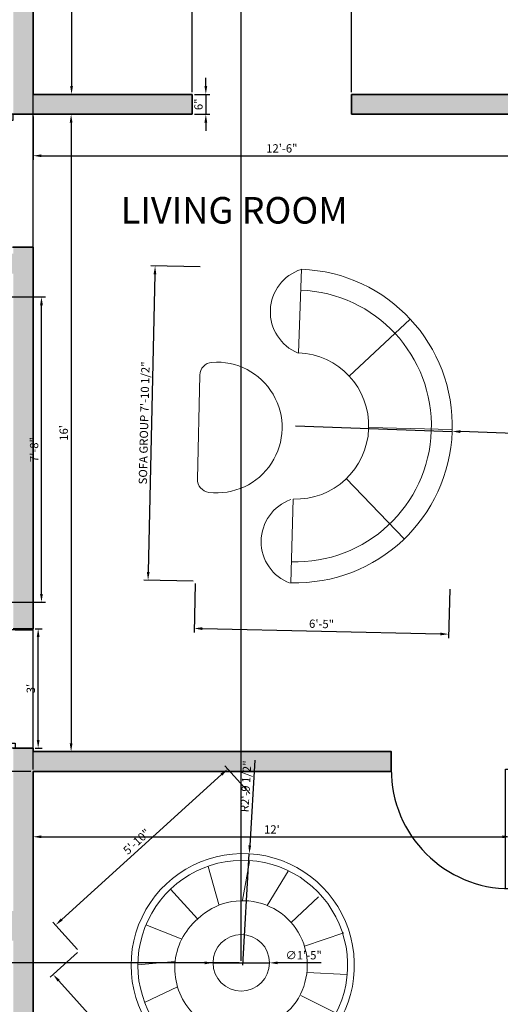
# Model space of a CAD drawing. Units: inches. Extents: x 2901 to 5923, y 918 to 2827.
# Tile 10 of 16: x 4585 to 4730, y 1227 to 1524. Entities that reach past the tile are written whole.
import ezdxf

# ---------------------------------------------------------------- set-up
doc = ezdxf.new("R2010")
doc.units = ezdxf.units.IN
for name, color, linetype, lineweight in [('A-ANNO-DIMS', 2, 'Continuous', 18), ('A-AREA-IDEN', 7, 'Continuous', 25), ('A-FLOR-PATT', 252, 'Continuous', 13), ('A-WALL-PATT', 7, 'Continuous', 13), ('doors', 240, 'Continuous', 25), ('furniture', 160, 'Continuous', 18), ('walls', 7, 'Continuous', 35)]:
    doc.layers.add(name, color=color, linetype=linetype, lineweight=lineweight)
doc.styles.get("Standard").update_dxf_attribs({"font": 'arial.ttf'})
doc.dimstyles.new('Copy of ISO-25', dxfattribs={"dimtxt": 2.5, "dimasz": 2.5, "dimexe": 1.25, "dimexo": 0.625, "dimtad": 1, "dimdec": 1, "dimlunit": 4, "dimtxsty": 'Standard', "dimcen": 2.5, "dimadec": 0, "dimazin": 0, "dimtfac": 1, "dimtdec": 1, "dimtmove": 0, "dimatfit": 3, "dimfxl": 1, "dimarcsym": 0})

# ---------------------------------------------------------------- blocks, each defined once
blk = doc.blocks.new('*U9')
for p, q in [((-40, 0), (-40, 6)), ((0, 0), (0, 6))]:
    blk.add_line(p, q)
blk.add_lwpolyline([(0, 0), (0, -40), (-1.75, -40), (-1.75, 0)], close=True)
blk.add_arc((0, 0), 40, 180, 270)
blk = doc.blocks.new('*U5')
for p, q in [((0, 0), (0, -6)), ((-40, 0), (-40, -6))]:
    blk.add_line(p, q)
blk.add_lwpolyline([(0, 0), (0, 40), (-1.75, 40), (-1.75, 0)], close=True)
blk.add_arc((0, 0), 40, 90, 180)
blk = doc.blocks.new('*U6')
for p, q in [((0, 0), (0, -6)), ((40, 0), (40, -6))]:
    blk.add_line(p, q)
blk.add_lwpolyline([(0, 0), (0, 40), (1.75, 40), (1.75, 0)], close=True)
blk.add_arc((0, 0), 40, 0, 90)
blk = doc.blocks.new('A$C22FC404C')
for p, q in [((1199.9, 1301.9), (1199.9, 1941.9)), ((809.2, 1143.1), (362.7, 1601.6)), ((1594.3, 1139.4), (2045.1, 1593.7)), ((0, 760.4), (639.9, 750.6)), ((2399.8, 731.4), (1759.8, 735.4)), ((827.3, 0), (1623.4, 0))]:
    blk.add_line(p, q)
for centre, radius, start, end in [((1199.9, 741.9), 1200, 359.49903, 179.11736), ((1199.9, 741.9), 1040, 359.40957, 179.11736), ((1199.9, 741.9), 560, 359.32862, 179.11736), ((323.1, 869.6), 340.6, 199.13086, 339.10386), ((2082.3, 838.8), 340.6, 200.89614, 340.86914), ((1225.3, 139.3), 500, 354.35827, 185.64173), ((827.3, 100), 100, 185.64173, 270), ((1623.4, 100), 100, 270, 354.35827)]:
    blk.add_arc(centre, radius, start, end)
blk = doc.blocks.new('A$C0ECE726C')
for p, q in [((1694, 2620), (1694, 3331)), ((1322, 2571), (1110, 3122)), ((1023, 2382), (606, 2799)), ((787, 2067), (221, 2311)), ((701, 1673), (142, 1666)), ((2687, 1673), (3320, 1664)), ((795, 1248), (221, 1075)), ((2593, 1248), (3113, 1091)), ((1016, 941), (551, 587)), ((2372, 941), (2811, 607)), ((1315, 753), (1055, 225)), ((2073, 753), (2322, 247)), ((1694, 100), (1694, 697))]:
    blk.add_line(p, q)
blk.add_circle((1652, 1618), 420)
for centre, radius, start, end in [((1660, 1660), 1660, 88.7606, 0.1441), ((1660, 1660), 1560, 88.7606, 0.2051), ((1392, 2970), 462, 310.7368, 49.2632), ((1660, 1660), 960, 87.986, 272.014), ((3002, 1543), 340, 20.831, 157.5545), ((1728, 1660), 960, 267.986, 0.781)]:
    blk.add_arc(centre, radius, start, end)
blk = doc.blocks.new('*D38')
at = {"layer": 'A-ANNO-DIMS', "color": 0, "lineweight": -2, "transparency": 16777216}
for p, q in [((4589.69, 1621.4), (4601.92, 1621.4)), ((4600.67, 1618.9), (4600.67, 1503.9)), ((4589.69, 1501.4), (4601.92, 1501.4))]:
    blk.add_line(p, q, dxfattribs=at)
at = {"layer": 'A-ANNO-DIMS', "color": 0, "transparency": 16777216}
for points in [[(4600.25, 1618.9), (4601.08, 1618.9), (4600.67, 1621.4)], [(4600.25, 1503.9), (4601.08, 1503.9), (4600.67, 1501.4)]]:
    blk.add_solid(points, dxfattribs=at)
at = {"layer": 'Defpoints', "color": 0, "transparency": 16777216}
for p in [(4589.07, 1621.4), (4589.07, 1501.4), (4600.67, 1501.4)]:
    blk.add_point(p, dxfattribs=at)
at = {"layer": 'A-ANNO-DIMS', "color": 0, "transparency": 16777216, "insert": (4598.76, 1561.4), "char_height": 2.5, "attachment_point": 5, "rotation": 90}
blk.add_mtext("10'", dxfattribs=at)
blk = doc.blocks.new('*D43')
at = {"layer": 'A-ANNO-DIMS', "color": 0, "lineweight": -2, "transparency": 16777216}
for p, q in [((4589.69, 1340.4), (4591.85, 1340.4)), ((4590.6, 1306.9), (4590.6, 1337.9)), ((4589.69, 1304.4), (4591.85, 1304.4))]:
    blk.add_line(p, q, dxfattribs=at)
at = {"layer": 'A-ANNO-DIMS', "color": 0, "transparency": 16777216}
for points in [[(4590.18, 1337.9), (4591.02, 1337.9), (4590.6, 1340.4)], [(4590.18, 1306.9), (4591.02, 1306.9), (4590.6, 1304.4)]]:
    blk.add_solid(points, dxfattribs=at)
at = {"layer": 'Defpoints', "color": 0, "transparency": 16777216}
for p in [(4589.07, 1340.4), (4590.6, 1340.4), (4589.07, 1304.4)]:
    blk.add_point(p, dxfattribs=at)
at = {"layer": 'A-ANNO-DIMS', "color": 0, "transparency": 16777216, "insert": (4588.7, 1322.4), "char_height": 2.5, "attachment_point": 5, "rotation": 90}
blk.add_mtext("3'", dxfattribs=at)
blk = doc.blocks.new('*D50')
at = {"layer": 'A-ANNO-DIMS', "color": 0, "lineweight": -2, "transparency": 16777216}
for p, q in [((4641.15, 1503.9), (4641.15, 1506.4)), ((4637.69, 1501.4), (4642.4, 1501.4)), ((4641.15, 1501.4), (4641.15, 1495.4)), ((4637.69, 1495.4), (4642.4, 1495.4)), ((4641.15, 1492.9), (4641.15, 1490.4))]:
    blk.add_line(p, q, dxfattribs=at)
at = {"layer": 'A-ANNO-DIMS', "color": 0, "transparency": 16777216}
for points in [[(4640.73, 1503.9), (4641.56, 1503.9), (4641.15, 1501.4)], [(4640.73, 1492.9), (4641.56, 1492.9), (4641.15, 1495.4)]]:
    blk.add_solid(points, dxfattribs=at)
at = {"layer": 'Defpoints', "color": 0, "transparency": 16777216}
for p in [(4637.07, 1501.4), (4637.07, 1495.4), (4641.15, 1495.4)]:
    blk.add_point(p, dxfattribs=at)
at = {"layer": 'A-ANNO-DIMS', "color": 0, "transparency": 16777216, "insert": (4639.25, 1498.4), "char_height": 2.5, "attachment_point": 5, "rotation": 90}
blk.add_mtext('6"', dxfattribs=at)
blk = doc.blocks.new('*D55')
at = {"layer": 'A-ANNO-DIMS', "color": 0, "lineweight": -2, "transparency": 16777216}
for p, q in [((4589.69, 1495.4), (4601.79, 1495.4)), ((4600.54, 1492.9), (4600.54, 1305.9)), ((4589.69, 1303.4), (4601.79, 1303.4))]:
    blk.add_line(p, q, dxfattribs=at)
at = {"layer": 'A-ANNO-DIMS', "color": 0, "transparency": 16777216}
for points in [[(4600.12, 1492.9), (4600.95, 1492.9), (4600.54, 1495.4)], [(4600.12, 1305.9), (4600.95, 1305.9), (4600.54, 1303.4)]]:
    blk.add_solid(points, dxfattribs=at)
at = {"layer": 'Defpoints', "color": 0, "transparency": 16777216}
for p in [(4589.07, 1495.4), (4589.07, 1303.4), (4600.54, 1303.4)]:
    blk.add_point(p, dxfattribs=at)
at = {"layer": 'A-ANNO-DIMS', "color": 0, "transparency": 16777216, "insert": (4598.63, 1399.4), "char_height": 2.5, "attachment_point": 5, "rotation": 90}
blk.add_mtext("16'", dxfattribs=at)
blk = doc.blocks.new('*D56')
at = {"layer": 'A-ANNO-DIMS', "color": 0, "lineweight": -2, "transparency": 16777216}
for p, q in [((4589.07, 1494.77), (4589.07, 1481.66)), ((4739.07, 1494.77), (4739.07, 1481.66)), ((4591.57, 1482.91), (4736.57, 1482.91))]:
    blk.add_line(p, q, dxfattribs=at)
at = {"layer": 'A-ANNO-DIMS', "color": 0, "transparency": 16777216}
for points in [[(4591.57, 1483.32), (4591.57, 1482.49), (4589.07, 1482.91)], [(4736.57, 1483.32), (4736.57, 1482.49), (4739.07, 1482.91)]]:
    blk.add_solid(points, dxfattribs=at)
at = {"layer": 'Defpoints', "color": 0, "transparency": 16777216}
for p in [(4589.07, 1495.4), (4739.07, 1495.4), (4739.07, 1482.91)]:
    blk.add_point(p, dxfattribs=at)
at = {"layer": 'A-ANNO-DIMS', "color": 0, "transparency": 16777216, "insert": (4664.07, 1484.81), "char_height": 2.5, "attachment_point": 5}
blk.add_mtext('12\'-6"', dxfattribs=at)
blk = doc.blocks.new('*D62')
at = {"layer": 'A-ANNO-DIMS', "color": 0, "lineweight": -2, "transparency": 16777216}
for p, q in [((4589.07, 1296.77), (4589.07, 1276.48)), ((4733.07, 1296.77), (4733.07, 1276.48)), ((4591.57, 1277.73), (4730.57, 1277.73))]:
    blk.add_line(p, q, dxfattribs=at)
at = {"layer": 'A-ANNO-DIMS', "color": 0, "transparency": 16777216}
for points in [[(4591.57, 1278.14), (4591.57, 1277.31), (4589.07, 1277.73)], [(4730.57, 1278.14), (4730.57, 1277.31), (4733.07, 1277.73)]]:
    blk.add_solid(points, dxfattribs=at)
at = {"layer": 'Defpoints', "color": 0, "transparency": 16777216}
for p in [(4589.07, 1297.4), (4733.07, 1297.4), (4733.07, 1277.73)]:
    blk.add_point(p, dxfattribs=at)
at = {"layer": 'A-ANNO-DIMS', "color": 0, "transparency": 16777216, "insert": (4661.07, 1279.61), "char_height": 2.5, "attachment_point": 5}
blk.add_mtext("12'", dxfattribs=at)
blk = doc.blocks.new('*D80')
at = {"layer": 'A-ANNO-DIMS', "color": 0, "lineweight": -2, "transparency": 16777216}
for p, q in [((4574.98, 1440.35), (4592.85, 1440.35)), ((4591.6, 1350.88), (4591.6, 1437.85)), ((4574.98, 1348.38), (4592.85, 1348.38))]:
    blk.add_line(p, q, dxfattribs=at)
at = {"layer": 'A-ANNO-DIMS', "color": 0, "transparency": 16777216}
for points in [[(4591.18, 1437.85), (4592.02, 1437.85), (4591.6, 1440.35)], [(4591.18, 1350.88), (4592.02, 1350.88), (4591.6, 1348.38)]]:
    blk.add_solid(points, dxfattribs=at)
at = {"layer": 'Defpoints', "color": 0, "transparency": 16777216}
for p in [(4574.36, 1440.35), (4591.6, 1440.35), (4574.36, 1348.38)]:
    blk.add_point(p, dxfattribs=at)
at = {"layer": 'A-ANNO-DIMS', "color": 0, "transparency": 16777216, "insert": (4589.7, 1394.37), "char_height": 2.5, "attachment_point": 5, "rotation": 90}
blk.add_mtext('7\'-8"', dxfattribs=at)
blk = doc.blocks.new('*D83')
at = {"layer": 'A-ANNO-DIMS', "color": 0, "lineweight": -2, "transparency": 16777216}
for p, q in [((4639.44, 1449.4), (4624.61, 1449.73)), ((4625.81, 1447.2), (4623.79, 1357.52)), ((4637.31, 1354.71), (4622.48, 1355.05))]:
    blk.add_line(p, q, dxfattribs=at)
at = {"layer": 'A-ANNO-DIMS', "color": 0, "transparency": 16777216}
for points in [[(4625.39, 1447.21), (4626.22, 1447.19), (4625.86, 1449.7)], [(4623.37, 1357.53), (4624.21, 1357.51), (4623.73, 1355.02)]]:
    blk.add_solid(points, dxfattribs=at)
at = {"layer": 'Defpoints', "color": 0, "transparency": 16777216}
for p in [(4640.07, 1449.38), (4623.73, 1355.02), (4637.94, 1354.7)]:
    blk.add_point(p, dxfattribs=at)
at = {"layer": 'A-ANNO-DIMS', "color": 0, "transparency": 16777216, "insert": (4622.88, 1402.4), "char_height": 2.5, "attachment_point": 5, "rotation": 88.7102}
blk.add_mtext('SOFA GROUP 7\'-10 1/2"', dxfattribs=at)
blk = doc.blocks.new('*D84')
at = {"layer": 'A-ANNO-DIMS', "color": 0, "lineweight": -2, "transparency": 16777216}
for p, q in [((4637.92, 1354.07), (4637.59, 1339.25)), ((4714.67, 1352.35), (4714.33, 1337.52)), ((4640.11, 1340.44), (4711.86, 1338.82))]:
    blk.add_line(p, q, dxfattribs=at)
at = {"layer": 'A-ANNO-DIMS', "color": 0, "transparency": 16777216}
for points in [[(4640.12, 1340.86), (4640.11, 1340.02), (4637.62, 1340.5)], [(4711.87, 1339.24), (4711.85, 1338.41), (4714.36, 1338.77)]]:
    blk.add_solid(points, dxfattribs=at)
at = {"layer": 'Defpoints', "color": 0, "transparency": 16777216}
for p in [(4637.94, 1354.7), (4714.68, 1352.97), (4714.36, 1338.77)]:
    blk.add_point(p, dxfattribs=at)
at = {"layer": 'A-ANNO-DIMS', "color": 0, "transparency": 16777216, "insert": (4676.03, 1341.53), "char_height": 2.5, "attachment_point": 5, "rotation": 358.7102}
blk.add_mtext('6\'-5"', dxfattribs=at)
blk = doc.blocks.new('*D85')
at = {"layer": 'A-ANNO-DIMS', "color": 0, "lineweight": -2, "transparency": 16777216}
for p, q in [((4602.46, 1242.89), (4594.18, 1235.39)), ((4596.79, 1234.37), (4640.62, 1186)), ((4649.65, 1190.81), (4641.38, 1183.31))]:
    blk.add_line(p, q, dxfattribs=at)
at = {"layer": 'A-ANNO-DIMS', "color": 0, "transparency": 16777216}
for points in [[(4597.1, 1234.65), (4596.48, 1234.09), (4595.11, 1236.23)], [(4640.93, 1186.28), (4640.32, 1185.72), (4642.3, 1184.15)]]:
    blk.add_solid(points, dxfattribs=at)
at = {"layer": 'Defpoints', "color": 0, "transparency": 16777216}
for p in [(4602.92, 1243.31), (4650.11, 1191.23), (4642.3, 1184.15)]:
    blk.add_point(p, dxfattribs=at)
at = {"layer": 'A-ANNO-DIMS', "color": 0, "transparency": 16777216, "insert": (4620.13, 1211.48), "char_height": 2.5, "attachment_point": 5, "rotation": 312.1851}
blk.add_mtext('SEATING 5\'-10 1/2"', dxfattribs=at)
blk = doc.blocks.new('*D86')
at = {"layer": 'A-ANNO-DIMS', "color": 0, "lineweight": -2, "transparency": 16777216}
for p, q in [((4645.87, 1296.46), (4597.69, 1252.8)), ((4654.38, 1290.79), (4646.88, 1299.06)), ((4602.5, 1243.77), (4595, 1252.04))]:
    blk.add_line(p, q, dxfattribs=at)
at = {"layer": 'A-ANNO-DIMS', "color": 0, "transparency": 16777216}
for points in [[(4645.59, 1296.77), (4646.15, 1296.15), (4647.72, 1298.14)], [(4597.41, 1253.1), (4597.97, 1252.49), (4595.84, 1251.12)]]:
    blk.add_solid(points, dxfattribs=at)
at = {"layer": 'Defpoints', "color": 0, "transparency": 16777216}
for p in [(4654.8, 1290.32), (4595.84, 1251.12), (4602.92, 1243.31)]:
    blk.add_point(p, dxfattribs=at)
at = {"layer": 'A-ANNO-DIMS', "color": 0, "transparency": 16777216, "insert": (4620.5, 1276.03), "char_height": 2.5, "attachment_point": 5, "rotation": 42.1851}
blk.add_mtext('5\'-10"', dxfattribs=at)
blk = doc.blocks.new('*D89')
at = {"layer": 'A-ANNO-DIMS', "color": 0, "lineweight": -2, "transparency": 16777216}
for p, q in [((4892.69, 1630.4), (5055.73, 1630.4)), ((5054.48, 989.9), (5054.48, 1627.9)), ((4709.69, 987.4), (5055.73, 987.4))]:
    blk.add_line(p, q, dxfattribs=at)
at = {"layer": 'A-ANNO-DIMS', "color": 0, "transparency": 16777216}
for points in [[(5054.06, 1627.9), (5054.9, 1627.9), (5054.48, 1630.4)], [(5054.06, 989.9), (5054.9, 989.9), (5054.48, 987.4)]]:
    blk.add_solid(points, dxfattribs=at)
at = {"layer": 'Defpoints', "color": 0, "transparency": 16777216}
for p in [(4892.07, 1630.4), (5054.48, 1630.4), (4709.07, 987.4)]:
    blk.add_point(p, dxfattribs=at)
at = {"layer": 'A-ANNO-DIMS', "color": 0, "transparency": 16777216, "insert": (5052.58, 1308.9), "char_height": 2.5, "attachment_point": 5, "rotation": 90}
blk.add_mtext('53\'-7"', dxfattribs=at)
blk = doc.blocks.new('*D101')
at = {"layer": 'A-ANNO-DIMS', "color": 0, "lineweight": -2, "transparency": 16777216}
for p, q in [((4637.07, 1502.02), (4637.07, 1724.84)), ((4639.57, 1723.59), (4682.57, 1723.59)), ((4685.07, 1502.02), (4685.07, 1724.84))]:
    blk.add_line(p, q, dxfattribs=at)
at = {"layer": 'A-ANNO-DIMS', "color": 0, "transparency": 16777216}
for points in [[(4639.57, 1724.01), (4639.57, 1723.18), (4637.07, 1723.59)], [(4682.57, 1724.01), (4682.57, 1723.18), (4685.07, 1723.59)]]:
    blk.add_solid(points, dxfattribs=at)
at = {"layer": 'Defpoints', "color": 0, "transparency": 16777216}
for p in [(4685.07, 1723.59), (4637.07, 1501.4), (4685.07, 1501.4)]:
    blk.add_point(p, dxfattribs=at)
at = {"layer": 'A-ANNO-DIMS', "color": 0, "transparency": 16777216, "insert": (4661.07, 1725.49), "char_height": 2.5, "attachment_point": 5}
blk.add_mtext('4\'-0"', dxfattribs=at)
blk = doc.blocks.new('*D102')
at = {"layer": 'A-ANNO-DIMS', "color": 0, "lineweight": -2, "transparency": 16777216}
for p, q in [((4589.07, 1502.02), (4589.07, 1724.84)), ((4591.57, 1723.59), (4634.57, 1723.59)), ((4637.07, 1502.02), (4637.07, 1724.84))]:
    blk.add_line(p, q, dxfattribs=at)
at = {"layer": 'A-ANNO-DIMS', "color": 0, "transparency": 16777216}
for points in [[(4591.57, 1724.01), (4591.57, 1723.18), (4589.07, 1723.59)], [(4634.57, 1724.01), (4634.57, 1723.18), (4637.07, 1723.59)]]:
    blk.add_solid(points, dxfattribs=at)
at = {"layer": 'Defpoints', "color": 0, "transparency": 16777216}
for p in [(4637.07, 1723.59), (4589.07, 1501.4), (4637.07, 1501.4)]:
    blk.add_point(p, dxfattribs=at)
at = {"layer": 'A-ANNO-DIMS', "color": 0, "transparency": 16777216, "insert": (4613.07, 1725.49), "char_height": 2.5, "attachment_point": 5}
blk.add_mtext('4\'-0"', dxfattribs=at)
blk = doc.blocks.new('*D105')
at = {"layer": 'A-ANNO-DIMS', "color": 0, "lineweight": -2, "transparency": 16777216}
for p, q in [((4589.07, 1298.02), (4589.07, 1724.84)), ((4591.57, 1723.59), (4649.33, 1723.59)), ((4651.83, 1240.37), (4651.83, 1724.84))]:
    blk.add_line(p, q, dxfattribs=at)
at = {"layer": 'A-ANNO-DIMS', "color": 0, "transparency": 16777216}
for points in [[(4591.57, 1724.01), (4591.57, 1723.18), (4589.07, 1723.59)], [(4649.33, 1724.01), (4649.33, 1723.18), (4651.83, 1723.59)]]:
    blk.add_solid(points, dxfattribs=at)
at = {"layer": 'Defpoints', "color": 0, "transparency": 16777216}
for p in [(4651.83, 1723.59), (4589.07, 1297.4), (4651.83, 1239.74)]:
    blk.add_point(p, dxfattribs=at)
at = {"layer": 'A-ANNO-DIMS', "color": 0, "transparency": 16777216, "insert": (4620.45, 1725.5), "char_height": 2.5, "attachment_point": 5}
blk.add_mtext('5\'-3"', dxfattribs=at)
blk = doc.blocks.new('*D106')
at = {"layer": 'A-ANNO-DIMS', "color": 0, "lineweight": -2, "transparency": 16777216}
for p, q in [((4588.44, 1297.4), (4247.63, 1297.4)), ((4248.88, 1294.9), (4248.88, 1242.24)), ((4651.2, 1239.74), (4247.63, 1239.74))]:
    blk.add_line(p, q, dxfattribs=at)
at = {"layer": 'A-ANNO-DIMS', "color": 0, "transparency": 16777216}
for points in [[(4248.46, 1294.9), (4249.3, 1294.9), (4248.88, 1297.4)], [(4248.46, 1242.24), (4249.3, 1242.24), (4248.88, 1239.74)]]:
    blk.add_solid(points, dxfattribs=at)
at = {"layer": 'Defpoints', "color": 0, "transparency": 16777216}
for p in [(4589.07, 1297.4), (4248.88, 1239.74), (4651.83, 1239.74)]:
    blk.add_point(p, dxfattribs=at)
at = {"layer": 'A-ANNO-DIMS', "color": 0, "transparency": 16777216, "insert": (4246.96, 1268.57), "char_height": 2.5, "attachment_point": 5, "rotation": 90}
blk.add_mtext('4\'-9 1/2"', dxfattribs=at)
blk = doc.blocks.new('*D107')
at = {"layer": 'A-ANNO-DIMS', "color": 0, "lineweight": -2, "transparency": 16777216}
for p, q in [((4640.81, 1239.74), (4638.31, 1239.74)), ((4643.31, 1239.74), (4660.34, 1239.74)), ((4675.96, 1239.74), (4662.84, 1239.74))]:
    blk.add_line(p, q, dxfattribs=at)
at = {"layer": 'A-ANNO-DIMS', "color": 0, "transparency": 16777216}
for points in [[(4640.81, 1240.16), (4640.81, 1239.32), (4643.31, 1239.74)], [(4662.84, 1240.16), (4662.84, 1239.33), (4660.34, 1239.74)]]:
    blk.add_solid(points, dxfattribs=at)
at = {"layer": 'Defpoints', "color": 0, "transparency": 16777216}
for p in [(4643.31, 1239.74), (4660.34, 1239.74)]:
    blk.add_point(p, dxfattribs=at)
at = {"layer": 'A-ANNO-DIMS', "color": 0, "transparency": 16777216, "insert": (4670.65, 1241.71), "char_height": 2.5, "attachment_point": 5, "rotation": 0.002}
blk.add_mtext('∅1\'-5"', dxfattribs=at)
blk = doc.blocks.new('*D108')
at = {"layer": 'A-ANNO-DIMS', "color": 0, "lineweight": -2, "transparency": 16777216}
for p, q in [((4668.21, 1401.5), (4715.42, 1399.87)), ((4749.86, 1398.67), (4717.92, 1399.78))]:
    blk.add_line(p, q, dxfattribs=at)
at = {"layer": 'A-ANNO-DIMS', "color": 0, "transparency": 16777216}
blk.add_solid([(4717.94, 1400.2), (4717.91, 1399.36), (4715.42, 1399.87)], dxfattribs=at)
at = {"layer": 'Defpoints', "color": 0, "transparency": 16777216}
for p in [(4668.21, 1401.5), (4715.42, 1399.87)]:
    blk.add_point(p, dxfattribs=at)
at = {"layer": 'A-ANNO-DIMS', "color": 0, "transparency": 16777216, "insert": (4743.82, 1400.79), "char_height": 2.5, "attachment_point": 5, "rotation": 358.0189}
blk.add_mtext('R3\'-11"', dxfattribs=at)
blk = doc.blocks.new('*D109')
at = {"layer": 'A-ANNO-DIMS', "color": 0, "lineweight": -2, "transparency": 16777216}
for p, q in [((4655.92, 1300.81), (4654.4, 1275.1)), ((4652.28, 1239.01), (4654.26, 1272.61))]:
    blk.add_line(p, q, dxfattribs=at)
at = {"layer": 'A-ANNO-DIMS', "color": 0, "transparency": 16777216}
blk.add_solid([(4653.99, 1275.13), (4654.82, 1275.08), (4654.26, 1272.61)], dxfattribs=at)
at = {"layer": 'Defpoints', "color": 0, "transparency": 16777216}
for p in [(4654.26, 1272.61), (4652.28, 1239.01)]:
    blk.add_point(p, dxfattribs=at)
at = {"layer": 'A-ANNO-DIMS', "color": 0, "transparency": 16777216, "insert": (4653.53, 1292.88), "char_height": 2.5, "attachment_point": 5, "rotation": 86.6374}
blk.add_mtext('R2\'-9 1/2"', dxfattribs=at)

msp = doc.modelspace()

# ---------------------------------------------------------------- hatches: boundary and pattern name
at = {"layer": 'A-FLOR-PATT'}
h = msp.add_hatch(dxfattribs=at)
h.set_pattern_fill('ANSI32', color=256)
h.paths.add_polyline_path([(4883.07, 1621.4), (4739.07, 1621.4), (4739.07, 1564.39, -0.396616), (4774.43, 1529.97), (4774.46, 1529.97), (4774.46, 1528.4), (4883.07, 1528.4)])
h.paths.add_polyline_path([(4733.07, 1143.4), (4685.07, 1143.4), (4685.07, 1147.03), (4684.01, 1147.03), (4684.01, 1171.22, 0.413071), (4660.87, 1146.06, 0.412532), (4638.11, 1170.77), (4638.11, 1146.97), (4637.07, 1143.4), (4589.07, 1143.4), (4589.07, 1029.4), (4733.07, 1029.4)])
h.paths.add_polyline_path([(4620.35, 1086.26, -0.333335), (4622.56, 1084.04), (4622.56, 1084.04), (4712.62, 1084.04, -0.333335), (4714.84, 1086.26), (4718.53, 1086.26, -0.376086), (4721.48, 1084.04), (4721.48, 1062.64), (4721.48, 1041.23, -0.333387), (4718.96, 1039.01), (4714.84, 1039.01, -0.333335), (4712.62, 1041.23), (4712.62, 1041.23), (4622.56, 1041.23, -0.333335), (4620.35, 1039.01), (4616.66, 1039.01, -0.376086), (4613.71, 1041.23), (4613.71, 1062.63), (4613.71, 1084.04, -0.333387), (4616.23, 1086.26)], flags=16)
h.paths.add_polyline_path([(4638.8, 1084.04), (4643.23, 1078.14), (4678.67, 1078.14), (4687.53, 1084.04), (4687.53, 1071.49), (4718.53, 1067.06), (4718.53, 1062.64), (4718.53, 1058.21), (4687.53, 1053.78), (4687.53, 1041.23), (4678.67, 1047.13), (4643.23, 1047.13), (4638.8, 1041.23), (4638.8, 1062.63)], flags=0)
at = {"layer": 'A-WALL-PATT'}
h = msp.add_hatch(color=256, dxfattribs=at)
h.dxf.hatch_style = 1
h.paths.add_polyline_path([(4439.07, 1447.4), (4583.07, 1447.4), (4583.07, 1340.4), (4589.07, 1340.4), (4589.07, 1453.4), (4589.07, 1455.39), (4583.07, 1455.39), (4583.07, 1453.4), (4439.07, 1453.4), (4439.07, 1501.84), (4430.07, 1501.84), (4430.07, 1399.4), (4439.07, 1399.4)])
h.paths.add_polyline_path([(4439.07, 1621.4), (4487.07, 1621.4), (4487.07, 1630.4), (4430.07, 1630.4), (4430.07, 1561.84), (4439.07, 1561.84)])
h.paths.add_polyline_path([(4630.61, 1630.4), (4535.07, 1630.4), (4535.07, 1621.4), (4583.07, 1621.4), (4583.07, 1495.4), (4589.07, 1495.4), (4637.07, 1495.4), (4637.07, 1501.4), (4589.07, 1501.4), (4589.07, 1621.4), (4630.61, 1621.4)])
h.paths.add_polyline_path([(4892.07, 1630.4), (4690.61, 1630.4), (4690.61, 1621.4), (4733.07, 1621.4), (4733.07, 1564.4), (4739.07, 1564.4), (4739.07, 1621.4), (4883.07, 1621.4), (4883.07, 1528.4), (4739.07, 1528.4), (4733.07, 1528.4), (4733.07, 1501.4), (4685.07, 1501.4), (4685.07, 1495.4), (4739.07, 1495.4), (4739.07, 1519.4), (4787.07, 1519.4), (4787.07, 1423.4), (4739.07, 1423.4), (4739.07, 1456.67), (4733.07, 1456.67), (4733.07, 1340.4), (4739.07, 1340.4), (4739.07, 1417.4), (4787.07, 1417.4), (4793.07, 1417.4), (4793.07, 1423.4), (4793.07, 1519.4), (4883.07, 1519.4), (4883.07, 1482.87), (4892.07, 1482.87)])
h.paths.add_polyline_path([(4892.07, 1458.87), (4883.07, 1458.87), (4883.07, 1423.4), (4823.07, 1423.4), (4823.07, 1417.4), (4883.07, 1417.4), (4883.07, 1363.31), (4892.07, 1363.31)], flags=17)
h.paths.add_polyline_path([(4892.07, 1303.31), (4883.07, 1303.31), (4883.07, 1255.4), (4739.07, 1255.4), (4739.07, 1304.4), (4733.07, 1304.4), (4733.07, 1303.4), (4733.07, 1297.4), (4733.07, 1255.4), (4733.07, 1248.4), (4811.07, 1248.4), (4811.07, 1212.16), (4820.07, 1212.16), (4820.07, 1248.4), (4892.07, 1248.4)])
h.paths.add_polyline_path([(4820.07, 1182.16), (4811.07, 1182.16), (4811.07, 1152.4), (4685.07, 1152.4), (4685.07, 1147.03), (4685.07, 1143.4), (4733.07, 1143.4), (4811.07, 1143.4), (4814.07, 1143.4), (4820.07, 1143.4)])
h.paths.add_polyline_path([(4637.07, 1152.4), (4589.07, 1152.4), (4589.07, 1153.4), (4583.86, 1153.4), (4583.07, 1153.4), (4583.07, 1152.4), (4511.07, 1152.4), (4511.07, 1182.16), (4502.07, 1182.16), (4502.07, 1143.4), (4568.07, 1143.4), (4583.07, 1143.4), (4583.07, 1023.4), (4739.07, 1023.4), (4739.07, 1143.4), (4733.07, 1143.4), (4733.07, 1029.4), (4589.07, 1029.4), (4589.07, 1143.4), (4637.07, 1143.4), (4637.07, 1146.97)])
h.paths.add_polyline_path([(4511.07, 1246.4), (4583.07, 1246.4), (4583.07, 1188.4), (4589.07, 1188.4), (4589.07, 1246.4), (4589.07, 1248.4), (4589.07, 1255.4), (4589.07, 1297.4), (4697.07, 1297.4), (4697.07, 1303.4), (4589.07, 1303.4), (4589.07, 1304.4), (4583.07, 1304.4), (4583.07, 1255.4), (4439.07, 1255.4), (4439.07, 1261.4), (4439.07, 1351.4), (4430.07, 1351.4), (4430.07, 1252.4), (4430.07, 1246.4), (4439.07, 1246.4), (4487.07, 1246.4), (4502.07, 1246.4), (4502.07, 1212.16), (4511.07, 1212.16)])

# ---------------------------------------------------------------- linework, layer by layer
at = {"layer": 'walls'}
for p, q in [((4589.07, 1621.4), (4589.07, 1501.4)), ((4637.07, 1501.4), (4589.07, 1501.4)), ((4637.07, 1501.4), (4637.07, 1495.4)), ((4733.07, 1501.4), (4685.07, 1501.4)), ((4685.07, 1495.4), (4685.07, 1501.4)), ((4589.07, 1495.4), (4583.07, 1495.4)), ((4637.07, 1495.4), (4589.07, 1495.4)), ((4739.07, 1495.4), (4685.07, 1495.4)), ((4589.07, 1455.4), (4583.07, 1455.4)), ((4589.07, 1453.4), (4589.07, 1455.4)), ((4589.07, 1453.4), (4589.07, 1340.4)), ((4583.07, 1340.4), (4589.07, 1340.4)), ((4589.07, 1304.4), (4583.07, 1304.4)), ((4589.07, 1303.4), (4589.07, 1304.4)), ((4589.07, 1304.4), (4589.07, 1303.4)), ((4589.07, 1303.4), (4697.07, 1303.4)), ((4697.07, 1303.4), (4697.07, 1297.4)), ((4589.07, 1255.4), (4589.07, 1297.4)), ((4589.07, 1297.4), (4697.07, 1297.4)), ((4589.07, 1297.4), (4589.07, 1255.4)), ((4589.07, 1248.4), (4589.07, 1255.4)), ((4589.07, 1246.4), (4589.07, 1248.4)), ((4589.07, 1246.4), (4589.07, 1188.4))]:
    msp.add_line(p, q, dxfattribs=at)

# ---------------------------------------------------------------- block references
at = {"layer": 'doors', "rotation": 90}
for name, p, xscale, yscale, zscale in [('*U5', (4583.07, 1495.4), 1.000274864133266, 1.000274864133266, 1.000274864133266), ('*U6', (4583.71, 1304.4), 0.8930329219077385, 0.8930329219077385, 0.8930329219077385)]:
    msp.add_blockref(name, p, dxfattribs=dict(at, xscale=xscale, yscale=yscale, zscale=zscale))
at = {"layer": 'doors', "xscale": 0.9008637989409386, "yscale": 0.9008637989409386, "zscale": 0.9008637989409386}
msp.add_blockref('*U9', (4733.07, 1298.09), dxfattribs=at)
at = {"layer": 'furniture'}
for name, p, xscale, yscale, zscale, rotation in [('A$C22FC404C', (4640.07, 1449.38), 0.0393700787401575, 0.0393700787401575, 0.0393700787401575, 268.7102432669956), ('A$C0ECE726C', (4654.62, 1286.55), 0.0202717158456741, 0.0202717158456741, 0.0202717158456741, 222.1851155917294)]:
    msp.add_blockref(name, p, dxfattribs=dict(at, xscale=xscale, yscale=yscale, zscale=zscale, rotation=rotation))

# ---------------------------------------------------------------- texts
at = {"layer": 'A-AREA-IDEN'}
msp.add_text('LIVING ROOM', height=8, dxfattribs=at).set_placement((4615.46, 1462.47))

# ---------------------------------------------------------------- dimensions: what is measured, and where the dimension line sits
at = {"layer": 'A-ANNO-DIMS'}
for base, p1, p2, override, picture, middle in [((4637.07, 1723.59), (4589.07, 1501.4), (4637.07, 1501.4), {"dimdec": 1, "dimlfac": 1, "dimrnd": 0, "dimzin": 1, "dimdsep": 46, "dimlunit": 4, "dimfrac": 2}, '*D102', (4613.07, 1725.49)), ((4651.83, 1723.59), (4589.07, 1297.4), (4651.83, 1239.74), {"dimdec": 1, "dimlfac": 1, "dimrnd": 0, "dimzin": 1, "dimdsep": 46, "dimlunit": 4, "dimfrac": 2}, '*D105', (4620.45, 1725.5)), ((4685.07, 1723.59), (4637.07, 1501.4), (4685.07, 1501.4), {"dimdec": 1, "dimlfac": 1, "dimrnd": 0, "dimzin": 1, "dimdsep": 46, "dimlunit": 4, "dimfrac": 2}, '*D101', (4661.07, 1725.49)), ((4739.07, 1482.91), (4589.07, 1495.4), (4739.07, 1495.4), {"dimclrd": 0, "dimclre": 0, "dimclrt": 0}, '*D56', (4664.07, 1484.81)), ((4733.07, 1277.73), (4589.07, 1297.4), (4733.07, 1297.4), {"dimclrd": 0, "dimclre": 0, "dimclrt": 0}, '*D62', (4661.07, 1279.61))]:
    dim = msp.add_linear_dim(base=base, p1=p1, p2=p2, dimstyle='Copy of ISO-25', override=override, dxfattribs=at)
    dim.commit()
    dim.dimension.update_dxf_attribs({"geometry": picture, "text_midpoint": middle})
for base, p1, p2, angle, override, picture, middle in [((5054.48, 1630.4), (4709.07, 987.4), (4892.07, 1630.4), 90, {"dimdec": 1, "dimlfac": 1, "dimrnd": 0, "dimzin": 1, "dimdsep": 46, "dimlunit": 4, "dimfrac": 2}, '*D89', (5052.58, 1308.9)), ((4600.67, 1501.4), (4589.07, 1621.4), (4589.07, 1501.4), 90, {"dimclrd": 0, "dimclre": 0, "dimclrt": 0}, '*D38', (4598.76, 1561.4)), ((4641.15, 1495.4), (4637.07, 1501.4), (4637.07, 1495.4), 90, {"dimclrd": 0, "dimclre": 0, "dimclrt": 0}, '*D50', (4639.25, 1498.4)), ((4600.54, 1303.4), (4589.07, 1495.4), (4589.07, 1303.4), 90, {"dimclrd": 0, "dimclre": 0, "dimclrt": 0}, '*D55', (4598.63, 1399.4)), ((4591.6, 1440.35), (4574.36, 1348.38), (4574.36, 1440.35), 90, {"dimdec": 1, "dimlfac": 1, "dimrnd": 0, "dimzin": 1, "dimdsep": 46, "dimlunit": 4, "dimfrac": 2}, '*D80', (4589.7, 1394.37)), ((4714.36, 1338.77), (4637.94, 1354.7), (4714.68, 1352.97), 358.7102, {"dimdec": 1, "dimlfac": 1, "dimrnd": 0, "dimzin": 1, "dimdsep": 46, "dimlunit": 4, "dimfrac": 2}, '*D84', (4676.03, 1341.53)), ((4590.6, 1340.4), (4589.07, 1304.4), (4589.07, 1340.4), 90, {"dimclrd": 0, "dimclre": 0, "dimclrt": 0}, '*D43', (4588.7, 1322.4)), ((4248.88, 1239.74), (4589.07, 1297.4), (4651.83, 1239.74), 90, {"dimdec": 1, "dimlfac": 1, "dimrnd": 0, "dimzin": 1, "dimdsep": 46, "dimlunit": 4, "dimfrac": 2}, '*D106', (4246.96, 1268.57)), ((4595.84, 1251.12), (4654.8, 1290.32), (4602.92, 1243.31), 222.1851, {"dimdec": 1, "dimlfac": 1, "dimrnd": 0, "dimzin": 1, "dimdsep": 46, "dimlunit": 4, "dimfrac": 2}, '*D86', (4620.5, 1276.03))]:
    dim = msp.add_linear_dim(base=base, p1=p1, p2=p2, angle=angle, dimstyle='Copy of ISO-25', override=override, dxfattribs=at)
    dim.commit()
    dim.dimension.update_dxf_attribs({"geometry": picture, "text_midpoint": middle})
for base, p1, p2, angle, text, picture, middle in [((4623.73, 1355.02), (4640.07, 1449.38), (4637.94, 1354.7), 268.7102, 'SOFA GROUP <>', '*D83', (4622.88, 1402.4)), ((4642.3, 1184.15), (4602.92, 1243.31), (4650.11, 1191.23), 312.1851, 'SEATING <>', '*D85', (4620.13, 1211.48))]:
    dim = msp.add_linear_dim(base=base, p1=p1, p2=p2, angle=angle, text=text, dimstyle='Copy of ISO-25', override={"dimdec": 1, "dimlfac": 1, "dimrnd": 0, "dimzin": 1, "dimdsep": 46, "dimlunit": 4, "dimfrac": 2}, dxfattribs=at)
    dim.commit()
    dim.dimension.update_dxf_attribs({"geometry": picture, "text_midpoint": middle})
for center, mpoint, picture, middle in [((4668.21, 1401.5), (4715.42, 1399.87), '*D108', (4743.75, 1398.89)), ((4652.28, 1239.01), (4654.26, 1272.61), '*D109', (4655.44, 1292.77))]:
    dim = msp.add_radius_dim(center=center, mpoint=mpoint, dimstyle='Copy of ISO-25', override={"dimdec": 1, "dimlfac": 1, "dimrnd": 0, "dimzin": 1, "dimdsep": 46, "dimlunit": 4, "dimfrac": 2}, dxfattribs=at)
    dim.commit()
    dim.dimension.update_dxf_attribs({"geometry": picture, "text_midpoint": middle, "dimtype": 164})
dim = msp.add_diameter_dim_2p(p1=(4643.31, 1239.74), p2=(4660.34, 1239.74), dimstyle='Copy of ISO-25', override={"dimdec": 1, "dimlfac": 1, "dimrnd": 0, "dimzin": 1, "dimdsep": 46, "dimlunit": 4, "dimfrac": 2}, dxfattribs=at)
dim.commit()
dim.dimension.update_dxf_attribs({"geometry": '*D107', "text_midpoint": (4670.65, 1239.74)})

doc.saveas('drawing.dxf')
